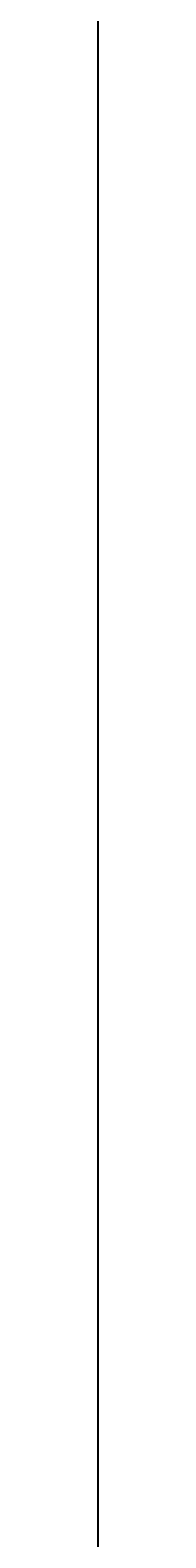
# Model space of a CAD drawing. Units: inches. Extents: x 2812 to 3051, y 1398 to 1659.
# Tile 12 of 65: x 2880 to 2880, y 1501 to 1528. Entities that reach past the tile are written whole.
import ezdxf

# ---------------------------------------------------------------- set-up
doc = ezdxf.new("R2010")
doc.units = ezdxf.units.IN
doc.layers.add('A-ANNO-DIMS', color=2, linetype='Continuous', lineweight=18)
doc.styles.get("Standard").update_dxf_attribs({"font": 'arial.ttf'})
doc.dimstyles.get("Standard").update_dxf_attribs({"dimtxt": 0.18, "dimasz": 0.18, "dimexe": 0.18, "dimexo": 0.0625, "dimgap": 0.09, "dimtad": 0, "dimtih": 1, "dimtoh": 1, "dimdec": 4, "dimzin": 0, "dimdsep": 46, "dimtxsty": 'Standard', "dimcen": 0.09, "dimadec": 0, "dimazin": 0, "dimtfac": 1, "dimtdec": 4, "dimtofl": 0, "dimtmove": 0, "dimatfit": 3, "dimfxl": 1, "dimtolj": 1, "dimtzin": 0, "dimarcsym": 0})

# ---------------------------------------------------------------- blocks, each defined once
blk = doc.blocks.new('*D58')
at = {"layer": 'A-ANNO-DIMS', "color": 0, "lineweight": -2, "transparency": 16777216}
for p, q in [((2880.385, 1472.098), (2880.385, 1659.35)), ((2880.565, 1659.17), (2881.736, 1659.17)), ((2883.205, 1659.17), (2882.034, 1659.17)), ((2883.385, 1472.098), (2883.385, 1659.35))]:
    blk.add_line(p, q, dxfattribs=at)
at = {"layer": 'A-ANNO-DIMS', "color": 0, "transparency": 16777216}
for points in [[(2880.565, 1659.2), (2880.565, 1659.14), (2880.385, 1659.17)], [(2883.205, 1659.2), (2883.205, 1659.14), (2883.385, 1659.17)]]:
    blk.add_solid(points, dxfattribs=at)
at = {"layer": 'Defpoints', "color": 0, "transparency": 16777216}
for p in [(2883.385, 1659.17), (2880.385, 1472.035), (2883.385, 1472.035)]:
    blk.add_point(p, dxfattribs=at)
at = {"layer": 'A-ANNO-DIMS', "color": 0, "transparency": 16777216, "insert": (2881.885, 1659.17), "char_height": 0.18, "attachment_point": 5}
blk.add_mtext('\\A1;3', dxfattribs=at)

msp = doc.modelspace()

# ---------------------------------------------------------------- dimensions: what is measured, and where the dimension line sits
at = {"layer": 'A-ANNO-DIMS'}
dim = msp.add_linear_dim(base=(2883.3849, 1659.17), p1=(2880.3849, 1472.0354), p2=(2883.3849, 1472.0354), dimstyle='Standard', override={"dimdec": 0, "dimlfac": 1, "dimrnd": 0, "dimzin": 0, "dimdsep": 46, "dimlunit": 2}, dxfattribs=at)
dim.commit()
dim.dimension.update_dxf_attribs({"geometry": '*D58', "text_midpoint": (2881.8849, 1659.17)})

doc.saveas('drawing.dxf')
